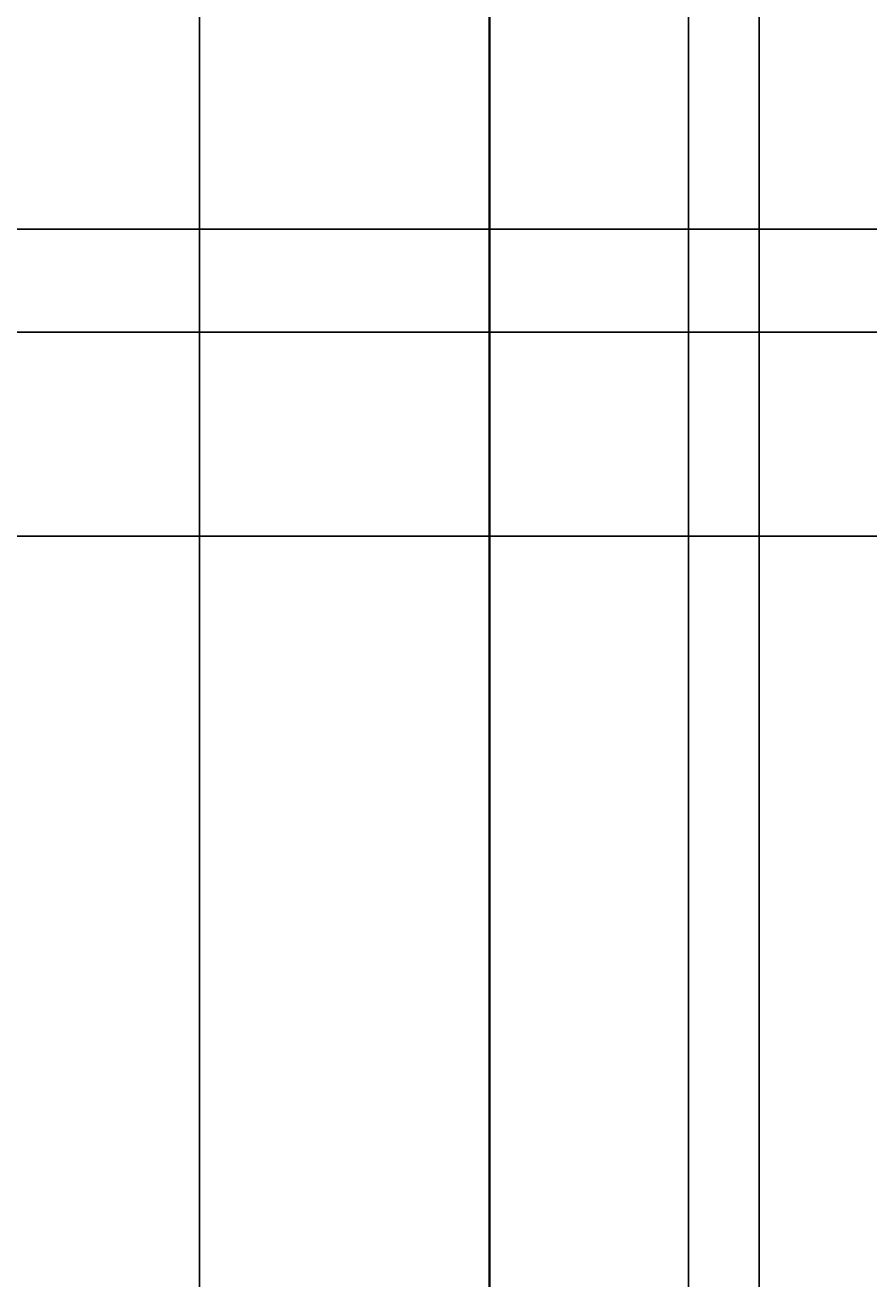
# Model space of a CAD drawing. Units: inches. Extents: x -6 to 289, y -8 to 323.
# Tile 24 of 107: x 102 to 126, y 87 to 124. Entities that reach past the tile are written whole.
import ezdxf

# ---------------------------------------------------------------- set-up
doc = ezdxf.new("R2010")
doc.units = ezdxf.units.IN
doc.header["$MEASUREMENT"] = 0
doc.layers.add('A-ANNO-DIMS', color=2, linetype='Continuous', lineweight=18)
doc.layers.add('A-ELEV', color=7, linetype='Continuous', lineweight=35)
doc.styles.get("Standard").update_dxf_attribs({"font": 'arial.ttf'})
doc.dimstyles.get("Standard").update_dxf_attribs({"dimtxt": 0.18, "dimasz": 0.18, "dimexe": 0.18, "dimexo": 0.0625, "dimgap": 0.09, "dimtad": 0, "dimtih": 1, "dimtoh": 1, "dimdec": 4, "dimzin": 0, "dimdsep": 46, "dimtxsty": 'Standard', "dimcen": 0.09, "dimadec": 0, "dimazin": 0, "dimtfac": 1, "dimtdec": 4, "dimtofl": 0, "dimtmove": 0, "dimatfit": 3, "dimfxl": 1, "dimtolj": 1, "dimtzin": 0, "dimarcsym": 0})

# ---------------------------------------------------------------- blocks, each defined once
blk = doc.blocks.new('*D58')
at = {"layer": 'A-ANNO-DIMS', "color": 0, "lineweight": -2, "transparency": 16777216}
for p, q in [((106.634, 68.495), (106.634, 322.969)), ((106.814, 322.789), (114.479, 322.789)), ((122.914, 322.789), (115.249, 322.789)), ((123.094, 68.495), (123.094, 322.969))]:
    blk.add_line(p, q, dxfattribs=at)
at = {"layer": 'A-ANNO-DIMS', "color": 0, "transparency": 16777216}
for points in [[(106.814, 322.819), (106.814, 322.759), (106.634, 322.789)], [(122.914, 322.819), (122.914, 322.759), (123.094, 322.789)]]:
    blk.add_solid(points, dxfattribs=at)
at = {"layer": 'Defpoints', "color": 0, "transparency": 16777216}
for p in [(123.094, 322.789), (106.634, 68.432), (123.094, 68.432)]:
    blk.add_point(p, dxfattribs=at)
at = {"layer": 'A-ANNO-DIMS', "color": 0, "transparency": 16777216, "insert": (114.864, 322.789), "char_height": 0.18, "attachment_point": 5}
blk.add_mtext('\\A1;16.46', dxfattribs=at)
blk = doc.blocks.new('*D73')
at = {"layer": 'A-ANNO-DIMS', "color": 0, "lineweight": -2, "transparency": 16777216}
for p, q in [((121.008, 51.148), (121.008, 322.969)), ((121.188, 322.789), (127.697, 322.789)), ((135.116, 322.789), (128.607, 322.789)), ((135.296, 51.148), (135.296, 322.969))]:
    blk.add_line(p, q, dxfattribs=at)
at = {"layer": 'A-ANNO-DIMS', "color": 0, "transparency": 16777216}
for points in [[(121.188, 322.819), (121.188, 322.759), (121.008, 322.789)], [(135.116, 322.819), (135.116, 322.759), (135.296, 322.789)]]:
    blk.add_solid(points, dxfattribs=at)
at = {"layer": 'Defpoints', "color": 0, "transparency": 16777216}
for p in [(135.296, 322.789), (121.008, 51.085), (135.296, 51.085)]:
    blk.add_point(p, dxfattribs=at)
at = {"layer": 'A-ANNO-DIMS', "color": 0, "transparency": 16777216, "insert": (128.152, 322.789), "char_height": 0.18, "attachment_point": 5}
blk.add_mtext('\\A1;14.288', dxfattribs=at)
blk = doc.blocks.new('*D87')
at = {"layer": 'A-ANNO-DIMS', "color": 0, "lineweight": -2, "transparency": 16777216}
for p, q in [((142.233, 108.948), (-5.737, 108.948)), ((-5.557, 108.768), (-5.557, 92.641)), ((-5.557, 76.151), (-5.557, 92.277)), ((166.233, 75.971), (-5.737, 75.971))]:
    blk.add_line(p, q, dxfattribs=at)
at = {"layer": 'A-ANNO-DIMS', "color": 0, "transparency": 16777216}
for points in [[(-5.587, 108.768), (-5.527, 108.768), (-5.557, 108.948)], [(-5.587, 76.151), (-5.527, 76.151), (-5.557, 75.971)]]:
    blk.add_solid(points, dxfattribs=at)
at = {"layer": 'Defpoints', "color": 0, "transparency": 16777216}
for p in [(-5.557, 108.948), (142.296, 108.948), (166.296, 75.971)]:
    blk.add_point(p, dxfattribs=at)
at = {"layer": 'A-ANNO-DIMS', "color": 0, "transparency": 16777216, "insert": (-5.557, 92.459), "char_height": 0.18, "attachment_point": 5}
blk.add_mtext('\\A1;32.98', dxfattribs=at)
blk = doc.blocks.new('*D88')
at = {"layer": 'A-ANNO-DIMS', "color": 0, "lineweight": -2, "transparency": 16777216}
for p, q in [((138.233, 114.948), (-5.737, 114.948)), ((-5.557, 114.768), (-5.557, 112.13)), ((-5.557, 109.128), (-5.557, 111.766)), ((142.233, 108.948), (-5.737, 108.948))]:
    blk.add_line(p, q, dxfattribs=at)
at = {"layer": 'A-ANNO-DIMS', "color": 0, "transparency": 16777216}
for points in [[(-5.587, 114.768), (-5.527, 114.768), (-5.557, 114.948)], [(-5.587, 109.128), (-5.527, 109.128), (-5.557, 108.948)]]:
    blk.add_solid(points, dxfattribs=at)
at = {"layer": 'Defpoints', "color": 0, "transparency": 16777216}
for p in [(-5.557, 114.948), (138.296, 114.948), (142.296, 108.948)]:
    blk.add_point(p, dxfattribs=at)
at = {"layer": 'A-ANNO-DIMS', "color": 0, "transparency": 16777216, "insert": (-5.557, 111.948), "char_height": 0.18, "attachment_point": 5}
blk.add_mtext('\\A1;6', dxfattribs=at)
blk = doc.blocks.new('*D89')
at = {"layer": 'A-ANNO-DIMS', "color": 0, "lineweight": -2, "transparency": 16777216}
for p, q in [((135.233, 117.971), (-5.737, 117.971)), ((-5.557, 117.791), (-5.557, 116.641)), ((-5.557, 115.128), (-5.557, 116.277)), ((138.233, 114.948), (-5.737, 114.948))]:
    blk.add_line(p, q, dxfattribs=at)
at = {"layer": 'A-ANNO-DIMS', "color": 0, "transparency": 16777216}
for points in [[(-5.587, 117.791), (-5.527, 117.791), (-5.557, 117.971)], [(-5.587, 115.128), (-5.527, 115.128), (-5.557, 114.948)]]:
    blk.add_solid(points, dxfattribs=at)
at = {"layer": 'Defpoints', "color": 0, "transparency": 16777216}
for p in [(-5.557, 117.971), (135.296, 117.971), (138.296, 114.948)]:
    blk.add_point(p, dxfattribs=at)
at = {"layer": 'A-ANNO-DIMS', "color": 0, "transparency": 16777216, "insert": (-5.557, 116.459), "char_height": 0.18, "attachment_point": 5}
blk.add_mtext('\\A1;3.023', dxfattribs=at)

msp = doc.modelspace()

# ---------------------------------------------------------------- linework, layer by layer
at = {"layer": 'A-ELEV'}
msp.add_line((115.1638, 127.2888), (115.1638, 68.4322), dxfattribs=at)

# ---------------------------------------------------------------- dimensions: what is measured, and where the dimension line sits
at = {"layer": 'A-ANNO-DIMS'}
for base, p1, p2, override, picture, middle in [((123.094, 322.7888), (106.634, 68.4322), (123.094, 68.4322), {"dimdec": 2, "dimlfac": 1, "dimrnd": 0, "dimzin": 0, "dimdsep": 46, "dimlunit": 2}, '*D58', (114.864, 322.7888)), ((135.296, 322.7888), (121.008, 51.0851), (135.296, 51.0851), {"dimdec": 3, "dimlfac": 1, "dimrnd": 0, "dimzin": 0, "dimdsep": 46, "dimlunit": 2}, '*D73', (128.152, 322.7888))]:
    dim = msp.add_linear_dim(base=base, p1=p1, p2=p2, dimstyle='Standard', override=override, dxfattribs=at)
    dim.commit()
    dim.dimension.update_dxf_attribs({"geometry": picture, "text_midpoint": middle})
for base, p1, p2, override, picture, middle in [((-5.557, 117.9706), (138.296, 114.9477), (135.296, 117.9706), {"dimdec": 3, "dimlfac": 1, "dimrnd": 0, "dimzin": 0, "dimdsep": 46, "dimlunit": 2}, '*D89', (-5.557, 116.4592)), ((-5.557, 114.9477), (142.296, 108.9477), (138.296, 114.9477), {"dimdec": 0, "dimlfac": 1, "dimrnd": 0, "dimzin": 0, "dimdsep": 46, "dimlunit": 2}, '*D88', (-5.557, 111.9477)), ((-5.557, 108.9477), (166.296, 75.9706), (142.296, 108.9477), {"dimdec": 2, "dimlfac": 1, "dimrnd": 0, "dimzin": 0, "dimdsep": 46, "dimlunit": 2}, '*D87', (-5.557, 92.4592))]:
    dim = msp.add_linear_dim(base=base, p1=p1, p2=p2, angle=90, dimstyle='Standard', override=override, dxfattribs=at)
    dim.commit()
    dim.dimension.update_dxf_attribs({"geometry": picture, "text_midpoint": middle})

doc.saveas('drawing.dxf')
